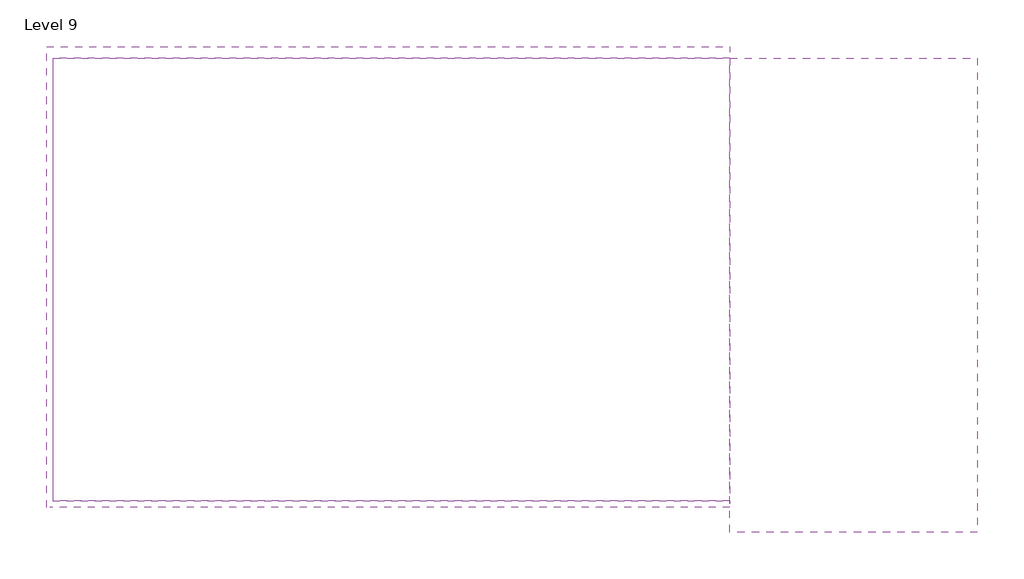
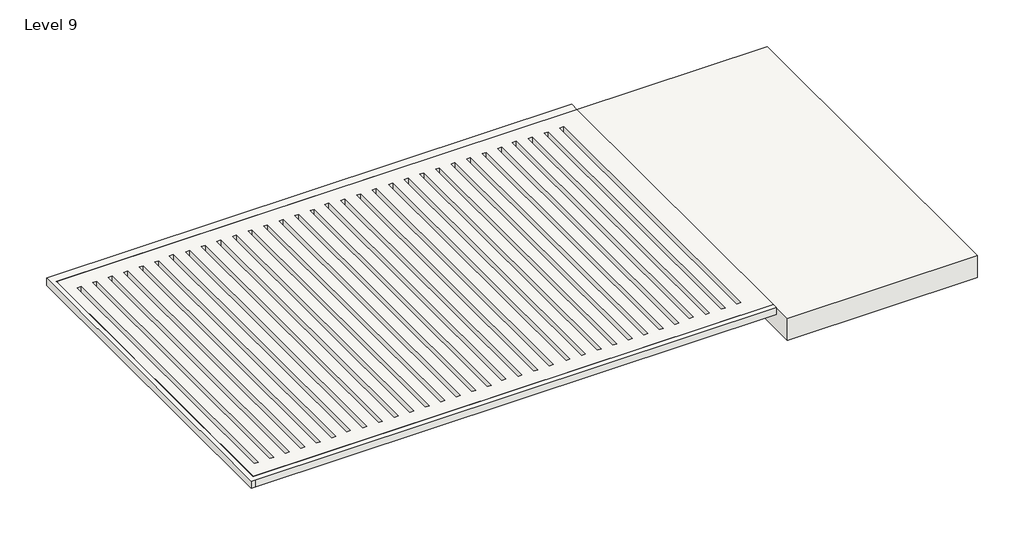
# One storey: 3 slabs.
"""IFC4 building model written with IfcOpenShell, lengths in millimetres."""

from ifc_helpers import new_model, si_unit, frame, origin, place, context, project, spatial, polyline, outline, extrude, element, save

model = new_model("IFC4")

# Units and contexts
model_context = context("Model", 3, world=origin())
ifc_project = project(units=[si_unit("LENGTHUNIT", "METRE", prefix="MILLI")], contexts=[model_context])

# Site, building, storey
site = spatial("IfcSite", under=ifc_project)
building = spatial("IfcBuilding", under=site)
storey = spatial("IfcBuildingStorey", under=building, Name="Level 9", Elevation=24384.0)

# Slabs
placement = place(None, origin())
element("IfcSlab", 1, ObjectType="Generic - 12\" 2", at=placement, inside=storey, context=model_context, shape_type="SweptSolid", body=[
    extrude(outline(polyline([(-25644.9874719, 12568.2170317), (-5234.0279391, 12568.2170317), (-5234.0279391, -784.3632813), (-25644.9874719, -784.3632813), (-25644.9874719, 12568.2170317)]), holes=[polyline([(-25076.8206231, 11899.8489683), (-25229.2206231, 11899.8489683), (-25229.2206231, -139.7510317), (-25076.8206231, -139.7510317), (-25076.8206231, 11899.8489683)]), polyline([(-24467.2206231, 11899.8489683), (-24619.6206231, 11899.8489683), (-24619.6206231, -139.7510317), (-24467.2206231, -139.7510317), (-24467.2206231, 11899.8489683)]), polyline([(-23857.6206231, 11899.8489683), (-24010.0206231, 11899.8489683), (-24010.0206231, -139.7510317), (-23857.6206231, -139.7510317), (-23857.6206231, 11899.8489683)]), polyline([(-22638.4206231, 11899.8489683), (-22790.8206231, 11899.8489683), (-22790.8206231, -139.7510317), (-22638.4206231, -139.7510317), (-22638.4206231, 11899.8489683)]), polyline([(-23248.0206231, 11899.8489683), (-23400.4206231, 11899.8489683), (-23400.4206231, -139.7510317), (-23248.0206231, -139.7510317), (-23248.0206231, 11899.8489683)]), polyline([(-22028.8206231, 11899.8489683), (-22181.2206231, 11899.8489683), (-22181.2206231, -139.7510317), (-22028.8206231, -139.7510317), (-22028.8206231, 11899.8489683)]), polyline([(-21419.7776933, 11963.6828901), (-21572.1776933, 11963.6828901), (-21572.1776933, -75.9171099), (-21419.7776933, -75.9171099), (-21419.7776933, 11963.6828901)]), polyline([(-20820.5561537, 11899.8489683), (-20972.9561537, 11899.8489683), (-20972.9561537, -139.7510317), (-20820.5561537, -139.7510317), (-20820.5561537, 11899.8489683)]), polyline([(-20200.0206231, 11899.8489683), (-20352.4206231, 11899.8489683), (-20352.4206231, -139.7510317), (-20200.0206231, -139.7510317), (-20200.0206231, 11899.8489683)]), polyline([(-19590.4206231, 11899.8489683), (-19742.8206231, 11899.8489683), (-19742.8206231, -139.7510317), (-19590.4206231, -139.7510317), (-19590.4206231, 11899.8489683)]), polyline([(-18980.8206231, 11899.8489683), (-19133.2206231, 11899.8489683), (-19133.2206231, -139.7510317), (-18980.8206231, -139.7510317), (-18980.8206231, 11899.8489683)]), polyline([(-18371.2206231, 11899.8489683), (-18523.6206231, 11899.8489683), (-18523.6206231, -139.7510317), (-18371.2206231, -139.7510317), (-18371.2206231, 11899.8489683)]), polyline([(-17761.6206231, 11899.8489683), (-17914.0206231, 11899.8489683), (-17914.0206231, -139.7510317), (-17761.6206231, -139.7510317), (-17761.6206231, 11899.8489683)]), polyline([(-16542.4206231, 11899.8489683), (-16694.8206231, 11899.8489683), (-16694.8206231, -139.7510317), (-16542.4206231, -139.7510317), (-16542.4206231, 11899.8489683)]), polyline([(-17152.0206231, 11899.8489683), (-17304.4206231, 11899.8489683), (-17304.4206231, -139.7510317), (-17152.0206231, -139.7510317), (-17152.0206231, 11899.8489683)]), polyline([(-15932.8206231, 11899.8489683), (-16085.2206231, 11899.8489683), (-16085.2206231, -139.7510317), (-15932.8206231, -139.7510317), (-15932.8206231, 11899.8489683)]), polyline([(-15323.7776933, 11963.6828901), (-15476.1776933, 11963.6828901), (-15476.1776933, -75.9171099), (-15323.7776933, -75.9171099), (-15323.7776933, 11963.6828901)]), polyline([(-14724.5561537, 11899.8489683), (-14876.9561537, 11899.8489683), (-14876.9561537, -139.7510317), (-14724.5561537, -139.7510317), (-14724.5561537, 11899.8489683)]), polyline([(-14104.0206231, 11899.8489683), (-14256.4206231, 11899.8489683), (-14256.4206231, -139.7510317), (-14104.0206231, -139.7510317), (-14104.0206231, 11899.8489683)]), polyline([(-13494.4206231, 11899.8489683), (-13646.8206231, 11899.8489683), (-13646.8206231, -139.7510317), (-13494.4206231, -139.7510317), (-13494.4206231, 11899.8489683)]), polyline([(-12843.3874719, 11899.8489683), (-12995.7874719, 11899.8489683), (-12995.7874719, -139.7510317), (-12843.3874719, -139.7510317), (-12843.3874719, 11899.8489683)]), polyline([(-12233.7874719, 11899.8489683), (-12386.1874719, 11899.8489683), (-12386.1874719, -139.7510317), (-12233.7874719, -139.7510317), (-12233.7874719, 11899.8489683)]), polyline([(-11624.1874719, 11899.8489683), (-11776.5874719, 11899.8489683), (-11776.5874719, -139.7510317), (-11624.1874719, -139.7510317), (-11624.1874719, 11899.8489683)]), polyline([(-11014.5874719, 11899.8489683), (-11166.9874719, 11899.8489683), (-11166.9874719, -139.7510317), (-11014.5874719, -139.7510317), (-11014.5874719, 11899.8489683)]), polyline([(-10404.9874719, 11899.8489683), (-10557.3874719, 11899.8489683), (-10557.3874719, -139.7510317), (-10404.9874719, -139.7510317), (-10404.9874719, 11899.8489683)]), polyline([(-9185.7874719, 11899.8489683), (-9338.1874719, 11899.8489683), (-9338.1874719, -139.7510317), (-9185.7874719, -139.7510317), (-9185.7874719, 11899.8489683)]), polyline([(-9795.3874719, 11899.8489683), (-9947.7874719, 11899.8489683), (-9947.7874719, -139.7510317), (-9795.3874719, -139.7510317), (-9795.3874719, 11899.8489683)]), polyline([(-8576.1874719, 11899.8489683), (-8728.5874719, 11899.8489683), (-8728.5874719, -139.7510317), (-8576.1874719, -139.7510317), (-8576.1874719, 11899.8489683)]), polyline([(-7967.1445421, 11963.6828901), (-8119.5445421, 11963.6828901), (-8119.5445421, -75.9171099), (-7967.1445421, -75.9171099), (-7967.1445421, 11963.6828901)]), polyline([(-7367.9230025, 11899.8489683), (-7520.3230025, 11899.8489683), (-7520.3230025, -139.7510317), (-7367.9230025, -139.7510317), (-7367.9230025, 11899.8489683)]), polyline([(-6747.3874719, 11899.8489683), (-6899.7874719, 11899.8489683), (-6899.7874719, -139.7510317), (-6747.3874719, -139.7510317), (-6747.3874719, 11899.8489683)]), polyline([(-6137.7874719, 11899.8489683), (-6290.1874719, 11899.8489683), (-6290.1874719, -139.7510317), (-6137.7874719, -139.7510317), (-6137.7874719, 11899.8489683)])]), frame((0.0, 0.0, 26517.6), z_axis=(0.0, 0.0, 1.0), x_axis=(1.0, 0.0, 0.0)), (0.0, 0.0, 1.0), 304.8),
])
element("IfcSlab", 2, ObjectType="Generic - 12\" 3", at=placement, inside=storey, context=model_context, shape_type="SweptSolid", body=[
    extrude(outline(polyline([(-25657.6874719, -784.3632813), (-5234.0279391, -784.3632813), (-5234.0279391, -987.5632813), (-25657.6874719, -987.5632813), (-25841.8374719, -987.5632813), (-25841.8374719, 12920.4712606), (-5234.0279391, 12920.4712606), (-5234.0279391, 12568.2170317), (-25657.6874719, 12568.2170317), (-25657.6874719, -784.3632813)])), frame((0.0, 0.0, 26517.6), z_axis=(0.0, 0.0, 1.0), x_axis=(1.0, 0.0, 0.0)), (0.0, 0.0, 1.0), 304.8),
])
element("IfcSlab", 3, ObjectType="Generic - 3'", at=placement, inside=storey, context=model_context, shape_type="SweptSolid", body=[
    extrude(outline(polyline([(2227.720997, 12568.2170317), (2227.720997, -1734.479389), (-5234.0279391, -1734.479389), (-5234.0279391, 12568.2170317), (2227.720997, 12568.2170317)])), frame((0.0, 0.0, 25908.0), z_axis=(0.0, 0.0, 1.0), x_axis=(1.0, 0.0, 0.0)), (0.0, 0.0, 1.0), 914.4),
])

save(model, "model.ifc")

# Revit data of these elements
# Type "Generic - 12\" 2"
#   Assembly Code = "B1010"
#   Function = 0
#   Layers, outside or top first: 1' - 0" "Softwood, Lumber" (function 1)
# Type "Generic - 12\" 3"
#   Assembly Code = "B1010"
#   Function = 0
#   Layers, outside or top first: 1' - 0" "Tile, Mosaic, Gray" (function 1)
# Type "Generic - 3'"
#   Assembly Code = "B1010"
#   Function = 0
#   Layers, outside or top first: 3' - 0" "Parking Stripe" (function 1)
# Element 1 (IfcSlab, "Generic - 12\" 2")
#   built-in parameter 1001955 = 3.14159 (stored number, unit not read)
#   Height Offset From Level = 8' - 0"
#   Phase Created = New Construction
#   Materials on its faces: "Softwood, Lumber"
# Element 2 (IfcSlab, "Generic - 12\" 3")
#   built-in parameter 1001955 = 3.14159 (stored number, unit not read)
#   Height Offset From Level = 8' - 0"
#   Phase Created = New Construction
#   Materials on its faces: "Tile, Mosaic, Gray"
# Element 3 (IfcSlab, "Generic - 3'")
#   Height Offset From Level = 8' - 0"
#   Phase Created = New Construction
#   Materials on its faces: "Parking Stripe"
# Materials
#   "Softwood, Lumber": class "Wood", colour RGB 223 192 134, transparency 0, Description = "Pinus Echinata", Cost = 0
#   "Tile, Mosaic, Gray": class "Generic", colour RGB 127 127 127, transparency 0, Description = "Mosiac tile, gray", Cost = 0
#   "Parking Stripe": class "Paint", colour RGB 250 250 91, transparency 0, Cost = 0
